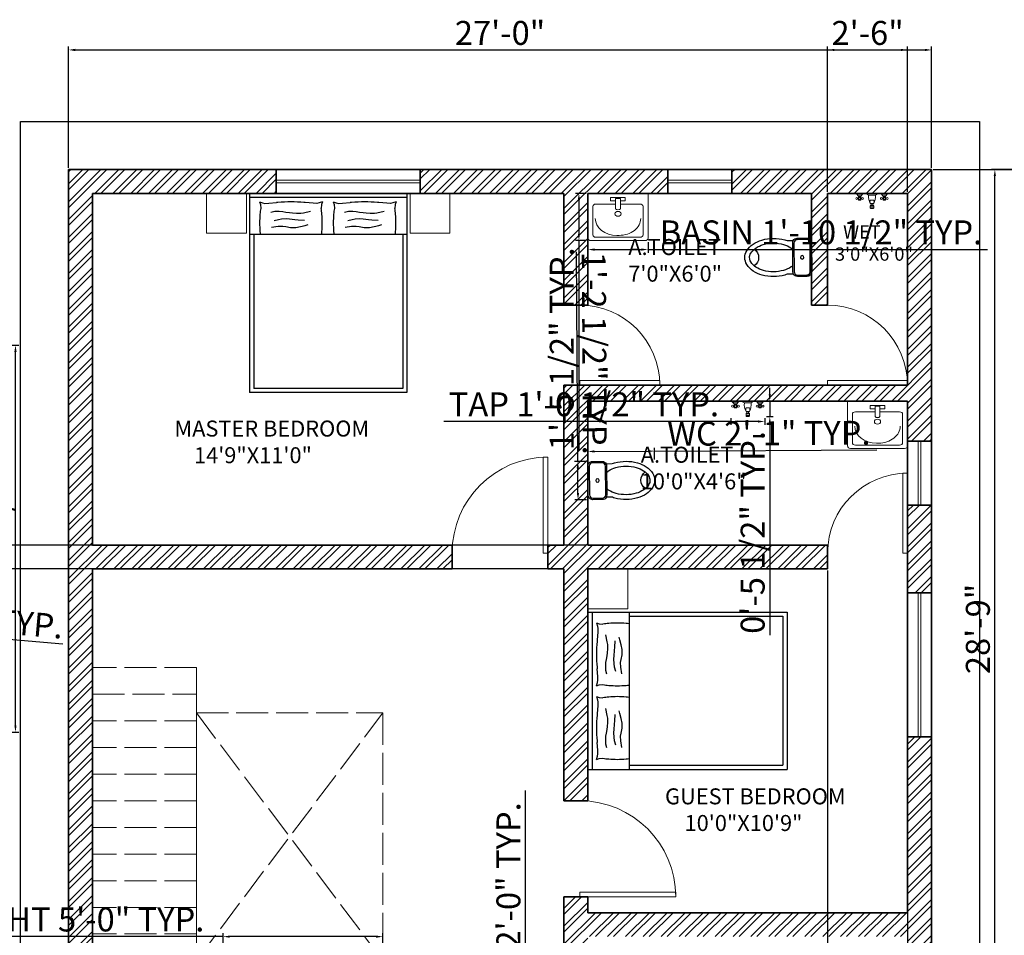
# Model space of a CAD drawing. Units: inches. Extents: x 638 to 1853, y 4393 to 5041.
# Tile 5 of 6: x 1072 to 1441, y 4619 to 4962. Entities that reach past the tile are written whole.
import ezdxf

# ---------------------------------------------------------------- set-up
doc = ezdxf.new("R2010")
doc.units = ezdxf.units.IN
doc.linetypes.add('ACAD_ISO02W100', pattern=[15, 12, -3])
for name, color, linetype, lineweight in [('A-ANNO-DIMS', 2, 'Continuous', 18), ('A-AREA-IDEN', 7, 'Continuous', 18), ('A-DOOR', 4, 'Continuous', 18), ('A-FLOR-FIXT', 9, 'Continuous', 18), ('A-FLOR-STRS', 7, 'Continuous', 18), ('A-FLOR-STRS-HIDN', 7, 'ACAD_ISO02W100', 18), ('A-FURN', 26, 'Continuous', 13), ('A-GLAZ', 5, 'Continuous', 18), ('A-WALL', 7, 'Continuous', 35), ('A-WALL-PATT', 251, 'Continuous', 13), ('C-PROP', 7, 'Continuous', 25)]:
    doc.layers.add(name, color=color, linetype=linetype, lineweight=lineweight)
for name, color, linetype in [('SANTEH', 7, 'Continuous'), ('supurgelik', 31, 'Continuous'), ('TASLAR', 32, 'Continuous')]:
    doc.layers.add(name, color=color, linetype=linetype)
doc.styles.get("Standard").update_dxf_attribs({"font": 'arial.ttf'})
doc.dimstyles.new('ISO-25', dxfattribs={"dimtxt": 9, "dimasz": 2.5, "dimexe": 1.25, "dimexo": 0.625, "dimtad": 1, "dimdec": 1, "dimlunit": 3, "dimtxsty": 'Standard', "dimcen": 2.5, "dimadec": 0, "dimazin": 0, "dimtfac": 1, "dimtdec": 1, "dimtmove": 0, "dimatfit": 3, "dimfxl": 1, "dimarcsym": 0})

# ---------------------------------------------------------------- blocks, each defined once
blk = doc.blocks.new('*U2')
for p, q in [((0, 0), (0, -6)), ((-36, 0), (-36, -6))]:
    blk.add_line(p, q)
blk.add_lwpolyline([(0, 0), (0, 36), (-1.75, 36), (-1.75, 0)], close=True)
blk.add_arc((0, 0), 36, 90, 180)
blk = doc.blocks.new('*U3')
for p, q in [((-30, 0), (-30, -6)), ((0, 0), (0, -6))]:
    blk.add_line(p, q)
blk.add_lwpolyline([(0, 0), (0, 30), (-1.75, 30), (-1.75, 0)], close=True)
blk.add_arc((0, 0), 30, 90, 180)
blk = doc.blocks.new('hgjgh')
at = {"layer": 'supurgelik'}
for p, q in [((85993.81, -4751.89), (85843.81, -4751.89)), ((85853.26, -4756.05), (85856.29, -4757)), ((85853.26, -4756.05), (85854.18, -4758.49)), ((85854.18, -4758.49), (85854.49, -4762.19)), ((85856.29, -4757), (85858.52, -4757.5)), ((85858.52, -4757.5), (85862.12, -4757.37)), ((85862.12, -4757.37), (85869.57, -4756.72)), ((85904.4, -4757.37), (85896.95, -4756.72)), ((85908, -4757.5), (85904.4, -4757.37)), ((85910.23, -4757), (85908, -4757.5)), ((85913.26, -4756.05), (85910.23, -4757)), ((85912.34, -4758.49), (85912.03, -4762.19)), ((85913.26, -4756.05), (85912.34, -4758.49)), ((85923.48, -4756.05), (85926.51, -4757)), ((85923.48, -4756.05), (85924.4, -4758.49)), ((85924.4, -4758.49), (85924.71, -4762.19)), ((85926.51, -4757), (85928.74, -4757.5)), ((85928.74, -4757.5), (85932.34, -4757.37)), ((85932.34, -4757.37), (85939.79, -4756.72)), ((85974.62, -4757.37), (85967.17, -4756.72)), ((85978.22, -4757.5), (85974.62, -4757.37)), ((85980.45, -4757), (85978.22, -4757.5)), ((85983.48, -4756.05), (85980.45, -4757)), ((85982.56, -4758.49), (85982.25, -4762.19)), ((85983.48, -4756.05), (85982.56, -4758.49)), ((85864.23, -4765.86), (85867.95, -4764.99)), ((85867.95, -4764.99), (85871.91, -4764.87)), ((85871.91, -4764.87), (85875.39, -4765.12)), ((85875.39, -4765.12), (85878.49, -4765.74)), ((85878.49, -4765.74), (85881.96, -4766.23)), ((85881.96, -4766.23), (85884.81, -4766.61)), ((85884.81, -4766.61), (85888.65, -4766.85)), ((85888.65, -4766.85), (85892.62, -4766.85)), ((85892.62, -4766.85), (85895.1, -4766.36)), ((85895.1, -4766.36), (85901.8, -4764.87)), ((85934.44, -4765.86), (85938.16, -4764.99)), ((85938.16, -4764.99), (85942.13, -4764.87)), ((85942.13, -4764.87), (85945.6, -4765.12)), ((85945.6, -4765.12), (85948.7, -4765.74)), ((85948.7, -4765.74), (85952.18, -4766.23)), ((85952.18, -4766.23), (85955.03, -4766.61)), ((85955.03, -4766.61), (85958.87, -4766.85)), ((85958.87, -4766.85), (85962.84, -4766.85)), ((85962.84, -4766.85), (85965.32, -4766.36)), ((85965.32, -4766.36), (85972.02, -4764.87)), ((85871.29, -4773.05), (85867.33, -4774.04)), ((85870.92, -4779.28), (85875.39, -4779.03)), ((85874.27, -4772.55), (85871.29, -4773.05)), ((85878.86, -4772.3), (85874.27, -4772.55)), ((85875.39, -4779.03), (85878.24, -4779.65)), ((85881.96, -4772.55), (85878.86, -4772.3)), ((85887.04, -4773.05), (85881.96, -4772.55)), ((85890.14, -4773.3), (85887.04, -4773.05)), ((85896.09, -4773.67), (85890.14, -4773.3)), ((85892.37, -4779.65), (85896.96, -4778.41)), ((85896.96, -4778.41), (85899.69, -4777.54)), ((85941.51, -4773.05), (85937.54, -4774.04)), ((85941.14, -4779.28), (85945.6, -4779.03)), ((85944.49, -4772.55), (85941.51, -4773.05)), ((85949.08, -4772.3), (85944.49, -4772.55)), ((85945.6, -4779.03), (85948.46, -4779.65)), ((85952.18, -4772.55), (85949.08, -4772.3)), ((85957.26, -4773.05), (85952.18, -4772.55)), ((85960.36, -4773.3), (85957.26, -4773.05)), ((85966.31, -4773.67), (85960.36, -4773.3)), ((85962.59, -4779.65), (85967.18, -4778.41)), ((85967.18, -4778.41), (85969.91, -4777.54)), ((85993.81, -4787.2), (85843.81, -4787.2)), ((85847.81, -4787.2), (85847.81, -4933.89)), ((85864.72, -4780.15), (85870.92, -4779.28)), ((85878.24, -4779.65), (85882.95, -4780.4)), ((85882.95, -4780.4), (85887.91, -4780.4)), ((85887.91, -4780.4), (85892.37, -4779.65)), ((85934.94, -4780.15), (85941.14, -4779.28)), ((85948.46, -4779.65), (85953.17, -4780.4)), ((85953.17, -4780.4), (85958.13, -4780.4)), ((85958.13, -4780.4), (85962.59, -4779.65)), ((85989.81, -4787.2), (85989.81, -4933.89)), ((85989.81, -4933.89), (85847.81, -4933.89))]:
    blk.add_line(p, q, dxfattribs=at)
for centre, radius, start, end in [((85877.36, -4828.49), 72.19, 95.13619, 96.19323), ((85883.26, -4894.18), 138.14, 90, 95.13619), ((85883.26, -4894.18), 138.14, 84.86381, 90), ((85889.16, -4828.49), 72.19, 83.80677, 84.86381), ((85947.57, -4828.49), 72.19, 95.13619, 96.19323), ((85953.48, -4894.18), 138.14, 90, 95.13619), ((85953.48, -4894.18), 138.14, 84.86381, 90), ((85959.38, -4828.49), 72.19, 83.80677, 84.86381), ((85954.09, -4776.05), 100.71, 175.30047, 180), ((85905.8, -4772.08), 52.26, 169.08956, 175.30047), ((85860.72, -4772.08), 52.26, 4.69953, 10.91044), ((85812.43, -4776.05), 100.71, 0, 4.69953), ((86024.31, -4776.05), 100.71, 175.30047, 180), ((85976.02, -4772.08), 52.26, 169.08956, 175.30047), ((85930.94, -4772.08), 52.26, 4.69953, 10.91044), ((85882.65, -4776.05), 100.71, 0, 4.69953), ((85954.09, -4776.05), 100.71, 180, 184.69953), ((85812.43, -4776.05), 100.71, 355.30047, 0), ((86024.31, -4776.05), 100.71, 180, 184.69953), ((85882.65, -4776.05), 100.71, 355.30047, 0), ((85905.8, -4780.02), 52.26, 184.69953, 187.89725), ((85860.72, -4780.02), 52.26, 352.10275, 355.30047), ((85976.02, -4780.02), 52.26, 184.69953, 187.89725), ((85930.94, -4780.02), 52.26, 352.10275, 355.30047)]:
    blk.add_arc(centre, radius, start, end, dxfattribs=at)
at = {"layer": 'TASLAR'}
for p, q in [((85843.81, -4747.89), (85843.81, -4937.89)), ((85993.81, -4747.89), (85843.81, -4747.89)), ((85993.81, -4747.89), (85993.81, -4937.89)), ((85993.81, -4937.89), (85843.81, -4937.89))]:
    blk.add_line(p, q, dxfattribs=at)
blk = doc.blocks.new('Rac7')
at = {"color": 0}
for p, q in [((-39500.6, -24232.1), (-39500.6, -23829.6)), ((-39473.6, -23808.4), (-38988.3, -23808.4)), ((-39456.5, -23859.1), (-39456.5, -24114.9)), ((-39032.4, -23838), (-39429.6, -23838)), ((-39221.1, -23854.9), (-39240.8, -23854.9)), ((-39005.4, -24114.9), (-39005.4, -23859.1)), ((-39005.4, -23859.1), (-39005.4, -23859.1)), ((-38961.3, -23829.6), (-38961.3, -24232.1)), ((-39252.5, -24185.9), (-39252.5, -24093.6)), ((-39209.4, -24185.9), (-39209.4, -24093.6)), ((-39429.6, -24136.1), (-39252.5, -24136.1)), ((-39297, -24164), (-39252.5, -24164)), ((-39297, -24193.5), (-39297, -24164)), ((-39164.9, -24193.5), (-39297, -24193.5)), ((-39252.5, -24185.9), (-39209.4, -24185.9)), ((-39209.4, -24136.1), (-39032.4, -24136.1)), ((-39209.4, -24164), (-39164.9, -24164)), ((-39164.9, -24164), (-39164.9, -24193.5)), ((-38961.3, -24232.1), (-39500.6, -24232.1))]:
    blk.add_line(p, q, dxfattribs=at)
at = {"color": 0, "extrusion": (0, 0, -1)}
for centre, major_axis, start_param, end_param in [((-39473.6, -23829.6), (-27, 0), 0, 1.570796), ((-39429.6, -23859.1), (-27, 0), 0, 1.570796), ((-39240.8, -24007.4), (-194.1, 0), 0, 1.570796), ((-39221.1, -24007.4), (-194.1, 0), 1.570796, 3.141593), ((-39032.4, -23859.1), (-27, 0), 1.570796, 3.141593), ((-38988.3, -23829.6), (-27, 0), 1.570796, 3.141593), ((-39429.6, -24114.9), (-27, 0), -1.570796, 0), ((-39231, -24104), (-25.3, 0), 0.552816, 2.588777), ((-39032.4, -24114.9), (-27, 0), -3.141593, -1.570796)]:
    blk.add_ellipse(centre, major_axis=major_axis, ratio=0.785714, start_param=start_param, end_param=end_param, dxfattribs=at)
blk.add_ellipse((-39231, -24048), major_axis=(-27.9, 0), ratio=0.785714, dxfattribs=at)
blk = doc.blocks.new('K10-44')
at = {"layer": 'SANTEH'}
for points in [[(-182, 223, 0.020439), (-174, 198), (-174, 135, 0.262987), (-198, 92), (-198, -8, 0.414214), (-148, -58), (152, -58, 0.414214), (202, -8), (202, 92, 0.262987), (178, 135), (178, 198, 0.020439), (186, 223, 0.067459), (202, 342, 0.067459), (186, 461, 0.079812), (143, 554, 0.107118), (74, 621, 0.139889), (2, 642, 0.139889), (-70, 621, 0.107118), (-140, 554, 0.079812), (-182, 461, 0.067459), (-198, 342, 0.067459)], [(-148, 127), (152, 127, -0.414214), (187, 92), (187, -8, -0.414214), (152, -43), (-148, -43, -0.414214), (-183, -8), (-183, 92, -0.414214)]]:
    blk.add_lwpolyline(points, format="xyb", close=True, dxfattribs=at)
for points in [[(90, 142, 0.027307), (102, 158, 0.079812), (137, 236, 0.067459), (152, 342, 0.067459), (137, 448, 0.079812), (102, 526, 0.107118), (47, 579, 0.139889), (2, 592, 0.139889), (-44, 579, 0.107118), (-98, 526, 0.079812), (-134, 448, 0.067459), (-148, 342, 0.067459), (-134, 236, 0.079812), (-98, 158, 0.027307), (-86, 142, 0.139889)], [(-174, 135, -0.136371), (-148, 142), (152, 142, -0.136371), (178, 135)]]:
    blk.add_lwpolyline(points, format="xyb", dxfattribs=at)
blk.add_circle((2, 42), 18.3, dxfattribs=at)
blk.add_arc((2, 602), 105, 213.8994, 326.1006, dxfattribs=at)
blk = doc.blocks.new('Faucet - Bathroom front')
for p, q in [((-0.5, 4.25), (0.5, 4.25)), ((0.5, 3.75), (-0.5, 3.75)), ((-0.5, 3), (0.5, 3)), ((-0.25, 3), (-0.25, 3.5)), ((0.25, 3.5), (0.25, 3)), ((-5, 0), (-2.25, 0)), ((-4.5087, 0.25), (-2.7408, 0.25)), ((-4, 1.625), (-4.25, 1.625)), ((-4, 1.375), (-4.25, 1.375)), ((-3.1442, 0.75), (-4.0979, 0.75)), ((-3.25, 1.625), (-3, 1.625)), ((-3.25, 1.375), (-3, 1.375)), ((-1.5, 0), (1.5, 0)), ((-1, 0.5), (1, 0.5)), ((0.5, 2), (-0.5, 2)), ((2.25, 0), (5, 0)), ((2.7413, 0.25), (4.5092, 0.25)), ((3.25, 1.625), (3, 1.625)), ((3.25, 1.375), (3, 1.375)), ((4.1058, 0.75), (3.1521, 0.75)), ((4, 1.625), (4.25, 1.625)), ((4, 1.375), (4.25, 1.375))]:
    blk.add_line(p, q)
for points in [[(-0.5, 3.75), (-0.5, 4.25)], [(-0.25, 4.5), (0.25, 4.5)], [(0.25, 3.5), (-0.25, 3.5)], [(0.5, 4.25), (0.5, 3.75)]]:
    blk.add_lwpolyline(points)
for points in [[(-4, 1), (-4, 2), (-3.25, 2), (-3.25, 1)], [(3.25, 1), (3.25, 2), (4, 2), (4, 1)]]:
    blk.add_lwpolyline(points, close=True)
for centre in [(-4.5, 1.5), (-3.625, 1.5), (-2.75, 1.5), (2.75, 1.5), (3.625, 1.5), (4.5, 1.5)]:
    blk.add_circle(centre, 0.2795)
for centre, radius, start, end in [((3, 1), 4.0311, 150.2551, 187.125), ((0.6413, 2.5), 1.246, 156.3417, 203.6583), ((-0.2575, 4.2575), 0.2426, 88.22243, 181.7776), ((-0.2575, 3.7425), 0.2426, 178.2224, 271.7776), ((0.2575, 4.2575), 0.2426, 358.2224, 91.77757), ((0.2575, 3.7425), 0.2426, 268.2224, 1.777565), ((-3, 1), 4.0311, 352.875, 29.74488), ((-0.6413, 2.5), 1.246, 336.3417, 23.65835), ((-5.375, 1.375), 1.4252, 285.2551, 344.7449), ((-1.875, 1.375), 1.4252, 195.2551, 254.7449), ((-0.7962, -0.2038), 0.7327, 106.1502, 163.8498), ((0.7962, -0.2038), 0.7327, 16.1502, 73.84979), ((1.875, 1.375), 1.4252, 285.2551, 344.7449), ((5.375, 1.375), 1.4252, 195.2551, 254.7449)]:
    blk.add_arc(centre, radius, start, end)
blk = doc.blocks.new('BED-NIGHTSTAND-15')
blk.add_lwpolyline([(0, 14.98), (14.98, 14.98), (14.98, 0), (0, 0)], close=True)
blk = doc.blocks.new('WINDOW-GLAZING-24IN')
for p, q in [((0, 24), (0, 0)), ((1, 24), (1, 0))]:
    blk.add_line(p, q)
blk = doc.blocks.new('WINDOW-GLAZING-54IN')
for p, q in [((0, 1), (54, 1)), ((0, 0), (54, 0))]:
    blk.add_line(p, q)
blk = doc.blocks.new('STAIR-WELL-OPENING')
for p, q in [((0, 93), (70, 0)), ((0, 0), (70, 93))]:
    blk.add_line(p, q)
blk.add_lwpolyline([(0, 93), (70, 93), (70, 0), (0, 0)], close=True)
blk = doc.blocks.new('STAIR-RUN-BEYOND')
for p, q in [((39, 100), (0, 100)), ((0, 90), (39, 90)), ((39, 80), (0, 80)), ((39, 70), (0, 70)), ((39, 60), (0, 60)), ((39, 50), (0, 50)), ((39, 40), (0, 40)), ((39, 30), (0, 30)), ((39, 20), (0, 20)), ((39, 10), (0, 10)), ((39, 0), (0, 0)), ((39, 0), (0, 0))]:
    blk.add_line(p, q)
blk = doc.blocks.new('*D40')
at = {"layer": 'A-ANNO-DIMS', "color": 0, "lineweight": -2, "transparency": 16777216}
for p, q in [((1285.04, 4797.16), (1285.01, 4801.55)), ((1287.52, 4800.31), (1307.62, 4800.43)), ((1310.13, 4797.3), (1310.11, 4801.69)), ((1310.12, 4800.44), (1393.53, 4800.92))]:
    blk.add_line(p, q, dxfattribs=at)
at = {"layer": 'A-ANNO-DIMS', "color": 0, "transparency": 16777216}
for points in [[(1287.52, 4800.73), (1287.52, 4799.9), (1285.02, 4800.3)], [(1307.61, 4800.84), (1307.62, 4800.01), (1310.12, 4800.44)]]:
    blk.add_solid(points, dxfattribs=at)
at = {"layer": 'Defpoints', "color": 0, "transparency": 16777216}
for p in [(1310.12, 4800.44), (1285.04, 4796.53), (1310.14, 4796.68)]:
    blk.add_point(p, dxfattribs=at)
at = {"layer": 'A-ANNO-DIMS', "color": 0, "transparency": 16777216, "insert": (1353.04, 4805.97), "char_height": 9, "attachment_point": 5, "rotation": 0.328}
blk.add_mtext('WC 2\'-1" TYP.', dxfattribs=at)
blk = doc.blocks.new('*D41')
at = {"layer": 'A-ANNO-DIMS', "color": 0, "lineweight": -2, "transparency": 16777216}
for p, q in [((1281.28, 4796.51), (1280.83, 4875.25)), ((1284.42, 4796.53), (1280.03, 4796.51)), ((1281.34, 4784.67), (1281.29, 4794.01)), ((1284.5, 4782.19), (1280.11, 4782.16))]:
    blk.add_line(p, q, dxfattribs=at)
at = {"layer": 'A-ANNO-DIMS', "color": 0, "transparency": 16777216}
for points in [[(1281.71, 4794.02), (1280.87, 4794.01), (1281.28, 4796.51)], [(1281.76, 4784.67), (1280.93, 4784.67), (1281.36, 4782.17)]]:
    blk.add_solid(points, dxfattribs=at)
at = {"layer": 'Defpoints', "color": 0, "transparency": 16777216}
for p in [(1281.28, 4796.51), (1285.04, 4796.53), (1285.12, 4782.19)]:
    blk.add_point(p, dxfattribs=at)
at = {"layer": 'A-ANNO-DIMS', "color": 0, "transparency": 16777216, "insert": (1286.32, 4837.16), "char_height": 9, "attachment_point": 5, "rotation": 270.328}
blk.add_mtext('1\'-2 1/2" TYP.', dxfattribs=at)
blk = doc.blocks.new('*D42')
at = {"layer": 'A-ANNO-DIMS', "color": 0, "lineweight": -2, "transparency": 16777216}
for p, q in [((1338.71, 4811.55), (1230.96, 4811.55)), ((1338.71, 4812.83), (1338.71, 4810.3)), ((1348.95, 4811.55), (1341.21, 4811.55)), ((1351.45, 4812.83), (1351.45, 4810.3))]:
    blk.add_line(p, q, dxfattribs=at)
at = {"layer": 'A-ANNO-DIMS', "color": 0, "transparency": 16777216}
for points in [[(1341.21, 4811.96), (1341.21, 4811.13), (1338.71, 4811.55)], [(1348.95, 4811.96), (1348.95, 4811.13), (1351.45, 4811.55)]]:
    blk.add_solid(points, dxfattribs=at)
at = {"layer": 'Defpoints', "color": 0, "transparency": 16777216}
for p in [(1338.71, 4813.46), (1351.45, 4813.46), (1338.71, 4811.55)]:
    blk.add_point(p, dxfattribs=at)
at = {"layer": 'A-ANNO-DIMS', "color": 0, "transparency": 16777216, "insert": (1283.58, 4816.83), "char_height": 9, "attachment_point": 5}
blk.add_mtext('TAP 1\'-0 1/2" TYP.', dxfattribs=at)
blk = doc.blocks.new('*D43')
at = {"layer": 'A-ANNO-DIMS', "color": 0, "lineweight": -2, "transparency": 16777216}
for p, q in [((1353.36, 4821.69), (1353.36, 4824.19)), ((1352.08, 4819.19), (1354.61, 4819.19)), ((1353.36, 4819.19), (1353.36, 4813.46)), ((1352.08, 4813.46), (1354.61, 4813.46)), ((1353.36, 4810.96), (1353.36, 4731.38))]:
    blk.add_line(p, q, dxfattribs=at)
at = {"layer": 'A-ANNO-DIMS', "color": 0, "transparency": 16777216}
for points in [[(1352.95, 4821.69), (1353.78, 4821.69), (1353.36, 4819.19)], [(1352.95, 4810.96), (1353.78, 4810.96), (1353.36, 4813.46)]]:
    blk.add_solid(points, dxfattribs=at)
at = {"layer": 'Defpoints', "color": 0, "transparency": 16777216}
for p in [(1351.45, 4819.19), (1351.45, 4813.46), (1353.36, 4813.46)]:
    blk.add_point(p, dxfattribs=at)
at = {"layer": 'A-ANNO-DIMS', "color": 0, "transparency": 16777216, "insert": (1348.09, 4769.92), "char_height": 9, "attachment_point": 5, "rotation": 90}
blk.add_mtext('0\'-5 1/2" TYP.', dxfattribs=at)
blk = doc.blocks.new('*D48')
at = {"layer": 'A-ANNO-DIMS', "color": 0, "lineweight": -2, "transparency": 16777216}
for p, q in [((1285.08, 4878.85), (1285.08, 4874.84)), ((1287.58, 4876.09), (1305.14, 4876.09)), ((1307.64, 4878.85), (1307.64, 4874.84)), ((1307.64, 4876.09), (1435.04, 4876.09))]:
    blk.add_line(p, q, dxfattribs=at)
at = {"layer": 'A-ANNO-DIMS', "color": 0, "transparency": 16777216}
for points in [[(1287.58, 4876.51), (1287.58, 4875.67), (1285.08, 4876.09)], [(1305.14, 4876.51), (1305.14, 4875.67), (1307.64, 4876.09)]]:
    blk.add_solid(points, dxfattribs=at)
at = {"layer": 'Defpoints', "color": 0, "transparency": 16777216}
for p in [(1285.08, 4879.47), (1307.64, 4879.47), (1307.64, 4876.09)]:
    blk.add_point(p, dxfattribs=at)
at = {"layer": 'A-ANNO-DIMS', "color": 0, "transparency": 16777216, "insert": (1372.59, 4881.37), "char_height": 9, "attachment_point": 5}
blk.add_mtext('BASIN 1\'-10 1/2" TYP.', dxfattribs=at)
blk = doc.blocks.new('*D49')
at = {"layer": 'A-ANNO-DIMS', "color": 0, "lineweight": -2, "transparency": 16777216}
for p, q in [((1284.46, 4897.19), (1280.45, 4897.19)), ((1281.7, 4894.69), (1281.7, 4881.97)), ((1284.46, 4879.47), (1280.45, 4879.47)), ((1281.7, 4879.47), (1281.7, 4800.74))]:
    blk.add_line(p, q, dxfattribs=at)
at = {"layer": 'A-ANNO-DIMS', "color": 0, "transparency": 16777216}
for points in [[(1281.28, 4894.69), (1282.11, 4894.69), (1281.7, 4897.19)], [(1281.28, 4881.97), (1282.11, 4881.97), (1281.7, 4879.47)]]:
    blk.add_solid(points, dxfattribs=at)
at = {"layer": 'Defpoints', "color": 0, "transparency": 16777216}
for p in [(1285.08, 4897.19), (1281.7, 4879.47), (1285.08, 4879.47)]:
    blk.add_point(p, dxfattribs=at)
at = {"layer": 'A-ANNO-DIMS', "color": 0, "transparency": 16777216, "insert": (1276.42, 4838.86), "char_height": 9, "attachment_point": 5, "rotation": 90}
blk.add_mtext('1\'-5 1/2" TYP.', dxfattribs=at)
blk = doc.blocks.new('*D51')
at = {"layer": 'A-ANNO-DIMS', "color": 0, "lineweight": -2, "transparency": 16777216}
for p, q in [((999.03, 4734.62), (999.24, 4737.06)), ((1001.62, 4735.59), (1006.2, 4735.19)), ((1008.59, 4733.79), (1008.8, 4736.22)), ((1008.69, 4734.98), (1087.97, 4728.04))]:
    blk.add_line(p, q, dxfattribs=at)
at = {"layer": 'A-ANNO-DIMS', "color": 0, "transparency": 16777216}
for points in [[(1001.66, 4736.01), (1001.59, 4735.18), (999.13, 4735.81)], [(1006.24, 4735.61), (1006.17, 4734.78), (1008.69, 4734.98)]]:
    blk.add_solid(points, dxfattribs=at)
at = {"layer": 'Defpoints', "color": 0, "transparency": 16777216}
for p in [(998.97, 4734), (1008.54, 4733.16), (1008.69, 4734.98)]:
    blk.add_point(p, dxfattribs=at)
at = {"layer": 'A-ANNO-DIMS', "color": 0, "transparency": 16777216, "insert": (1050.04, 4736.66), "char_height": 9, "attachment_point": 5, "rotation": 355}
blk.add_mtext('0\'-9 1/2" TYP.', dxfattribs=at)
blk = doc.blocks.new('*D56')
at = {"layer": 'A-ANNO-DIMS', "color": 0, "lineweight": -2, "transparency": 16777216}
for p, q in [((1261.68, 4538.69), (1261.68, 4673.01)), ((1258.71, 4538.69), (1262.93, 4538.69)), ((1261.68, 4517.19), (1261.68, 4536.19)), ((1258.71, 4514.69), (1262.93, 4514.69))]:
    blk.add_line(p, q, dxfattribs=at)
at = {"layer": 'A-ANNO-DIMS', "color": 0, "transparency": 16777216}
for points in [[(1261.26, 4536.19), (1262.1, 4536.19), (1261.68, 4538.69)], [(1261.26, 4517.19), (1262.1, 4517.19), (1261.68, 4514.69)]]:
    blk.add_solid(points, dxfattribs=at)
at = {"layer": 'Defpoints', "color": 0, "transparency": 16777216}
for p in [(1258.08, 4538.69), (1261.68, 4538.69), (1258.08, 4514.69)]:
    blk.add_point(p, dxfattribs=at)
at = {"layer": 'A-ANNO-DIMS', "color": 0, "transparency": 16777216, "insert": (1256.4, 4607.1), "char_height": 9, "attachment_point": 5, "rotation": 90}
blk.add_mtext('DOOR LEAF 2\'-0" TYP.', dxfattribs=at)
blk = doc.blocks.new('*D58')
at = {"layer": 'A-ANNO-DIMS', "color": 0, "lineweight": -2, "transparency": 16777216}
for p, q in [((1148.08, 4618.19), (1000.8, 4618.19)), ((1148.08, 4609.82), (1148.08, 4619.44)), ((1205.58, 4618.19), (1150.58, 4618.19)), ((1208.08, 4609.82), (1208.08, 4619.44))]:
    blk.add_line(p, q, dxfattribs=at)
at = {"layer": 'A-ANNO-DIMS', "color": 0, "transparency": 16777216}
for points in [[(1150.58, 4618.61), (1150.58, 4617.78), (1148.08, 4618.19)], [(1205.58, 4618.61), (1205.58, 4617.78), (1208.08, 4618.19)]]:
    blk.add_solid(points, dxfattribs=at)
at = {"layer": 'Defpoints', "color": 0, "transparency": 16777216}
for p in [(1148.08, 4618.19), (1148.08, 4609.19), (1208.08, 4609.19)]:
    blk.add_point(p, dxfattribs=at)
at = {"layer": 'A-ANNO-DIMS', "color": 0, "transparency": 16777216, "insert": (1073.19, 4623.47), "char_height": 9, "attachment_point": 5}
blk.add_mtext('STAIR FLIGHT 5\'-0" TYP.', dxfattribs=at)
blk = doc.blocks.new('*D83')
at = {"layer": 'A-ANNO-DIMS', "color": 0, "lineweight": -2, "transparency": 16777216}
for p, q in [((1016.97, 4840.19), (1071.42, 4840.19)), ((1070.17, 4697.42), (1070.17, 4837.69)), ((1016.97, 4694.92), (1071.42, 4694.92))]:
    blk.add_line(p, q, dxfattribs=at)
at = {"layer": 'A-ANNO-DIMS', "color": 0, "transparency": 16777216}
for points in [[(1069.75, 4837.69), (1070.58, 4837.69), (1070.17, 4840.19)], [(1069.75, 4697.42), (1070.58, 4697.42), (1070.17, 4694.92)]]:
    blk.add_solid(points, dxfattribs=at)
at = {"layer": 'Defpoints', "color": 0, "transparency": 16777216}
for p in [(1016.34, 4840.19), (1070.17, 4840.19), (1016.34, 4694.92)]:
    blk.add_point(p, dxfattribs=at)
at = {"layer": 'A-ANNO-DIMS', "color": 0, "transparency": 16777216, "insert": (1064.89, 4767.56), "char_height": 9, "attachment_point": 5, "rotation": 90}
blk.add_mtext('12\'-1 1/2"', dxfattribs=at)
blk = doc.blocks.new('*D88')
at = {"layer": 'A-ANNO-DIMS', "color": 0, "lineweight": -2, "transparency": 16777216}
for p, q in [((1090.08, 4906.82), (1090.08, 4952.27)), ((1092.58, 4951.02), (1411.58, 4951.02)), ((1414.08, 4906.82), (1414.08, 4952.27))]:
    blk.add_line(p, q, dxfattribs=at)
at = {"layer": 'A-ANNO-DIMS', "color": 0, "transparency": 16777216}
for points in [[(1092.58, 4951.44), (1092.58, 4950.6), (1090.08, 4951.02)], [(1411.58, 4951.44), (1411.58, 4950.6), (1414.08, 4951.02)]]:
    blk.add_solid(points, dxfattribs=at)
at = {"layer": 'Defpoints', "color": 0, "transparency": 16777216}
for p in [(1414.08, 4951.02), (1090.08, 4906.19), (1414.08, 4906.19)]:
    blk.add_point(p, dxfattribs=at)
at = {"layer": 'A-ANNO-DIMS', "color": 0, "transparency": 16777216, "insert": (1252.08, 4956.24), "char_height": 9, "attachment_point": 5}
blk.add_mtext('27\'-0"', dxfattribs=at)
blk = doc.blocks.new('*D89')
at = {"layer": 'A-ANNO-DIMS', "color": 0, "lineweight": -2, "transparency": 16777216}
for p, q in [((1414.71, 4906.19), (1460.16, 4906.19)), ((1458.91, 4458.69), (1458.91, 4903.69)), ((1414.71, 4456.19), (1460.16, 4456.19))]:
    blk.add_line(p, q, dxfattribs=at)
at = {"layer": 'A-ANNO-DIMS', "color": 0, "transparency": 16777216}
for points in [[(1458.49, 4903.69), (1459.32, 4903.69), (1458.91, 4906.19)], [(1458.49, 4458.69), (1459.32, 4458.69), (1458.91, 4456.19)]]:
    blk.add_solid(points, dxfattribs=at)
at = {"layer": 'Defpoints', "color": 0, "transparency": 16777216}
for p in [(1414.08, 4906.19), (1458.91, 4906.19), (1414.08, 4456.19)]:
    blk.add_point(p, dxfattribs=at)
at = {"layer": 'A-ANNO-DIMS', "color": 0, "transparency": 16777216, "insert": (1453.68, 4681.19), "char_height": 9, "attachment_point": 5, "rotation": 90}
blk.add_mtext('37\'-6"', dxfattribs=at)
blk = doc.blocks.new('*D91')
at = {"layer": 'A-ANNO-DIMS', "color": 0, "lineweight": -2, "transparency": 16777216}
for p, q in [((1375.08, 4897.82), (1375.08, 4952.27)), ((1377.58, 4951.02), (1402.58, 4951.02)), ((1405.08, 4897.82), (1405.08, 4952.27))]:
    blk.add_line(p, q, dxfattribs=at)
at = {"layer": 'A-ANNO-DIMS', "color": 0, "transparency": 16777216}
for points in [[(1377.58, 4951.44), (1377.58, 4950.6), (1375.08, 4951.02)], [(1402.58, 4951.44), (1402.58, 4950.6), (1405.08, 4951.02)]]:
    blk.add_solid(points, dxfattribs=at)
at = {"layer": 'Defpoints', "color": 0, "transparency": 16777216}
for p in [(1405.08, 4951.02), (1375.08, 4897.19), (1405.08, 4897.19)]:
    blk.add_point(p, dxfattribs=at)
at = {"layer": 'A-ANNO-DIMS', "color": 0, "transparency": 16777216, "insert": (1390.08, 4956.24), "char_height": 9, "attachment_point": 5}
blk.add_mtext('2\'-6"', dxfattribs=at)
blk = doc.blocks.new('*D92')
at = {"layer": 'A-ANNO-DIMS', "color": 0, "lineweight": -2, "transparency": 16777216}
for p, q in [((1375.08, 4755.57), (1375.08, 4416.12)), ((1405.08, 4755.57), (1405.08, 4416.12)), ((1377.58, 4417.37), (1402.58, 4417.37))]:
    blk.add_line(p, q, dxfattribs=at)
at = {"layer": 'A-ANNO-DIMS', "color": 0, "transparency": 16777216}
for points in [[(1377.58, 4417.79), (1377.58, 4416.95), (1375.08, 4417.37)], [(1402.58, 4417.79), (1402.58, 4416.95), (1405.08, 4417.37)]]:
    blk.add_solid(points, dxfattribs=at)
at = {"layer": 'Defpoints', "color": 0, "transparency": 16777216}
for p in [(1375.08, 4756.19), (1405.08, 4756.19), (1405.08, 4417.37)]:
    blk.add_point(p, dxfattribs=at)
at = {"layer": 'A-ANNO-DIMS', "color": 0, "transparency": 16777216, "insert": (1390.08, 4422.59), "char_height": 9, "attachment_point": 5}
blk.add_mtext('2\'-6"', dxfattribs=at)
blk = doc.blocks.new('*D93')
at = {"layer": 'A-ANNO-DIMS', "color": 0, "lineweight": -2, "transparency": 16777216}
for p, q in [((1045.26, 4765.19), (1045.26, 4792.87)), ((1284.46, 4765.19), (1044.01, 4765.19)), ((1045.26, 4758.69), (1045.26, 4762.69)), ((1275.46, 4756.19), (1044.01, 4756.19))]:
    blk.add_line(p, q, dxfattribs=at)
at = {"layer": 'A-ANNO-DIMS', "color": 0, "transparency": 16777216}
for points in [[(1044.84, 4762.69), (1045.67, 4762.69), (1045.26, 4765.19)], [(1044.84, 4758.69), (1045.67, 4758.69), (1045.26, 4756.19)]]:
    blk.add_solid(points, dxfattribs=at)
at = {"layer": 'Defpoints', "color": 0, "transparency": 16777216}
for p in [(1045.26, 4765.19), (1285.08, 4765.19), (1276.08, 4756.19)]:
    blk.add_point(p, dxfattribs=at)
at = {"layer": 'A-ANNO-DIMS', "color": 0, "transparency": 16777216, "insert": (1040.04, 4780.28), "char_height": 9, "attachment_point": 5, "rotation": 90}
blk.add_mtext('0\'-9"', dxfattribs=at)
blk = doc.blocks.new('*D97')
at = {"layer": 'A-ANNO-DIMS', "color": 0, "lineweight": -2, "transparency": 16777216}
for p, q in [((1482.06, 4906.19), (1436.61, 4906.19)), ((1437.86, 4563.69), (1437.86, 4903.69)), ((1482.06, 4561.19), (1436.61, 4561.19))]:
    blk.add_line(p, q, dxfattribs=at)
at = {"layer": 'A-ANNO-DIMS', "color": 0, "transparency": 16777216}
for points in [[(1437.44, 4903.69), (1438.27, 4903.69), (1437.86, 4906.19)], [(1437.44, 4563.69), (1438.27, 4563.69), (1437.86, 4561.19)]]:
    blk.add_solid(points, dxfattribs=at)
at = {"layer": 'Defpoints', "color": 0, "transparency": 16777216}
for p in [(1437.86, 4906.19), (1482.68, 4906.19), (1482.68, 4561.19)]:
    blk.add_point(p, dxfattribs=at)
at = {"layer": 'A-ANNO-DIMS', "color": 0, "transparency": 16777216, "insert": (1432.64, 4733.69), "char_height": 9, "attachment_point": 5, "rotation": 90}
blk.add_mtext('28\'-9"', dxfattribs=at)

msp = doc.modelspace()

# ---------------------------------------------------------------- hatches: boundary and pattern name
at = {"layer": 'A-WALL-PATT', "transparency": 33554687}
h = msp.add_hatch(dxfattribs=at)
h.set_pattern_fill('ANSI32', color=256, scale=0.5)
h.set_pattern_definition([(45, (-45.7406, 0), (-3.367596, 3.367596), []), (45, (-43.4956, 0), (-3.367596, 3.367596), [])])
h.paths.add_polyline_path([(1414.08, 4693.19), (1405.08, 4693.19), (1405.08, 4627.19), (1285.08, 4627.19), (1285.08, 4633.19), (1282.08, 4633.19), (1276.08, 4633.19), (1276.08, 4612.19), (1282.08, 4612.19), (1285.08, 4612.19), (1285.08, 4618.19), (1405.08, 4618.19), (1405.08, 4465.19), (1381.08, 4465.19), (1381.08, 4456.19), (1414.08, 4456.19)])
h.paths.add_polyline_path([(1216.08, 4519.19), (1156.08, 4519.19), (1156.08, 4531.19), (1150.08, 4531.19), (1147.08, 4531.19), (1147.08, 4465.19), (1099.08, 4465.19), (1099.08, 4474.19), (1090.08, 4474.19), (1090.08, 4456.19), (1156.08, 4456.19), (1156.08, 4510.19), (1216.08, 4510.19)])
h.paths.add_polyline_path([(1285.08, 4576.19), (1276.08, 4576.19), (1276.08, 4519.19), (1258.08, 4519.19), (1258.08, 4517.69), (1258.08, 4514.69), (1258.08, 4510.19), (1276.08, 4510.19), (1276.08, 4456.19), (1309.08, 4456.19), (1309.08, 4465.19), (1285.08, 4465.19)])
h.paths.add_polyline_path([(1414.08, 4780.19), (1405.08, 4780.19), (1405.08, 4762.19), (1405.08, 4756.19), (1405.08, 4747.19), (1414.08, 4747.19)], flags=17)
h.paths.add_polyline_path([(1414.08, 4906.19), (1339.08, 4906.19), (1339.08, 4897.19), (1369.08, 4897.19), (1369.08, 4855.19), (1375.08, 4855.19), (1375.08, 4897.19), (1405.08, 4897.19), (1405.08, 4825.19), (1276.08, 4825.19), (1276.08, 4765.19), (1270.08, 4765.19), (1270.08, 4756.19), (1276.08, 4756.19), (1276.08, 4669.19), (1285.08, 4669.19), (1285.08, 4756.19), (1375.08, 4756.19), (1375.08, 4765.19), (1285.08, 4765.19), (1285.08, 4819.19), (1405.08, 4819.19), (1405.08, 4804.19), (1414.08, 4804.19)])
h.paths.add_polyline_path([(1315.08, 4906.19), (1222.08, 4906.19), (1222.08, 4897.19), (1233.28, 4897.19), (1276.08, 4897.19), (1276.08, 4855.19), (1282.08, 4855.19), (1285.08, 4855.19), (1285.08, 4897.19), (1307.64, 4897.19), (1315.08, 4897.19)])
h.paths.add_polyline_path([(1099.08, 4897.19), (1168.08, 4897.19), (1168.08, 4906.19), (1090.08, 4906.19), (1090.08, 4498.19), (1099.08, 4498.19), (1099.08, 4561.19), (1115.92, 4561.19), (1210.08, 4561.19), (1210.08, 4570.19), (1099.08, 4570.19), (1099.08, 4756.19), (1234.08, 4756.19), (1234.08, 4762.19), (1234.08, 4765.19), (1099.08, 4765.19)])
h.paths.add_polyline_path([(1312.08, 4654.44), (1389.59, 4654.44), (1389.59, 4676.83), (1312.08, 4676.83)], flags=25)
h.paths.add_polyline_path([(1302.5, 4782.68), (1343.68, 4782.68), (1343.68, 4805.07), (1302.5, 4805.07)], flags=25)
h.paths.add_polyline_path([(1298.34, 4860.64), (1339, 4860.64), (1339, 4883.02), (1298.34, 4883.02)], flags=25)

# ---------------------------------------------------------------- linework, layer by layer
at = {"layer": 'A-FLOR-STRS'}
msp.add_line((1138.08, 4570.19), (1138.08, 4719.19), dxfattribs=at)
at = {"layer": 'A-WALL'}
for p, q in [((1090.08, 4906.19), (1414.08, 4906.19)), ((1090.08, 4456.19), (1090.08, 4906.19)), ((1168.08, 4897.19), (1168.08, 4906.19)), ((1222.08, 4897.19), (1222.08, 4906.19)), ((1315.08, 4897.19), (1315.08, 4906.19)), ((1339.08, 4897.19), (1339.08, 4906.19)), ((1414.08, 4906.19), (1414.08, 4456.19)), ((1099.08, 4897.19), (1276.08, 4897.19)), ((1099.08, 4765.19), (1099.08, 4897.19)), ((1276.08, 4855.19), (1276.08, 4897.19)), ((1285.08, 4897.19), (1369.08, 4897.19)), ((1285.08, 4855.19), (1285.08, 4897.19)), ((1369.08, 4897.19), (1369.08, 4855.19)), ((1375.08, 4897.19), (1375.08, 4855.19)), ((1375.08, 4897.19), (1405.08, 4897.19)), ((1405.08, 4897.19), (1405.08, 4825.19)), ((1276.08, 4855.19), (1285.08, 4855.19)), ((1369.08, 4855.19), (1375.08, 4855.19)), ((1276.08, 4825.19), (1405.08, 4825.19)), ((1276.08, 4765.19), (1276.08, 4825.19)), ((1285.08, 4819.19), (1405.08, 4819.19)), ((1285.08, 4765.19), (1285.08, 4819.19)), ((1405.08, 4819.19), (1405.08, 4627.19)), ((1405.08, 4804.19), (1414.08, 4804.19)), ((1405.08, 4780.19), (1414.08, 4780.19)), ((1099.08, 4765.19), (1234.08, 4765.19)), ((1234.08, 4756.19), (1234.08, 4765.19)), ((1270.08, 4765.19), (1276.08, 4765.19)), ((1270.08, 4756.19), (1270.08, 4765.19)), ((1285.08, 4765.19), (1375.08, 4765.19)), ((1375.08, 4765.19), (1375.08, 4756.19)), ((1099.08, 4756.19), (1234.08, 4756.19)), ((1099.08, 4570.19), (1099.08, 4756.19)), ((1270.08, 4756.19), (1276.08, 4756.19)), ((1276.08, 4669.19), (1276.08, 4756.19)), ((1285.08, 4756.19), (1375.08, 4756.19)), ((1285.08, 4669.19), (1285.08, 4756.19)), ((1405.08, 4747.19), (1414.08, 4747.19)), ((1405.08, 4693.19), (1414.08, 4693.19)), ((1285.08, 4669.19), (1276.08, 4669.19)), ((1276.08, 4612.19), (1276.08, 4633.19)), ((1285.08, 4633.19), (1276.08, 4633.19)), ((1285.08, 4627.19), (1285.08, 4633.19)), ((1405.08, 4627.19), (1285.08, 4627.19))]:
    msp.add_line(p, q, dxfattribs=at)
at = {"layer": 'C-PROP'}
msp.add_lwpolyline([(1072.08, 4924.19), (1432.08, 4924.19), (1432.08, 4444.19), (1072.08, 4444.19)], close=True, dxfattribs=at)

# ---------------------------------------------------------------- block references
at = {"layer": 'A-DOOR', "rotation": 270}
for name, p in [('*U3', (1282.08, 4825.19)), ('*U3', (1375.08, 4825.19)), ('*U2', (1282.08, 4633.19))]:
    msp.add_blockref(name, p, dxfattribs=at)
at = {"layer": 'A-DOOR'}
for name, p in [('*U2', (1270.08, 4762.19)), ('*U3', (1405.08, 4762.19))]:
    msp.add_blockref(name, p, dxfattribs=at)
at = {"layer": 'A-FLOR-FIXT'}
for name, p, xscale, yscale, zscale, rotation in [('Rac7', (2937.37, 3883.58), -0.0418294453001151, 0.0418294453001151, 0.0418294453001151, 180), ('Faucet - Bathroom front', (1391.73, 4897.19), 1.274234813154425, 1.274234813154425, 1.274234813154425, 180), ('K10-44', (1367, 4873.25), -0.0358529150226637, 0.0358529150226637, 0.0358529150226637, 90.3279556026283), ('Faucet - Bathroom front', (1345.08, 4819.19), 1.274234813154425, 1.274234813154425, 1.274234813154425, 180), ('Rac7', (3034.81, 3805.58), -0.0418294453001151, 0.0418294453001151, 0.0418294453001151, 180), ('K10-44', (1287.16, 4789.31), -0.0358529150226637, 0.0358529150226637, 0.0358529150226637, 270.3279556026283)]:
    msp.add_blockref(name, p, dxfattribs=dict(at, xscale=xscale, yscale=yscale, zscale=zscale, rotation=rotation))
at = {"layer": 'A-FLOR-STRS-HIDN'}
for name, p in [('STAIR-RUN-BEYOND', (1099.08, 4619.19)), ('STAIR-WELL-OPENING', (1138.08, 4609.19))]:
    msp.add_blockref(name, p, dxfattribs=at)
at = {"layer": 'A-FURN'}
for p in [(1141.89, 4882.21), (1218.29, 4882.21)]:
    msp.add_blockref('BED-NIGHTSTAND-15', p, dxfattribs=at)
at = {"layer": 'A-FURN', "xscale": 0.393701, "yscale": 0.393701, "zscale": 0.393701}
msp.add_blockref('hgjgh', (-32638.74, 6766.44), dxfattribs=at)
at = {"layer": 'A-FURN', "rotation": 90.00000000364122}
msp.add_blockref('BED-NIGHTSTAND-15', (1300.07, 4741.21), dxfattribs=at)
at = {"layer": 'A-FURN', "xscale": 0.393701, "yscale": 0.393701, "zscale": 0.393701, "rotation": 90}
msp.add_blockref('hgjgh', (-584.17, -29115.82), dxfattribs=at)
at = {"layer": 'A-GLAZ'}
for name, p, rotation in [('WINDOW-GLAZING-54IN', (1222.08, 4902.19), 180), ('WINDOW-GLAZING-24IN', (1315.08, 4902.19), 269.9999999999998), ('WINDOW-GLAZING-54IN', (1409.08, 4747.19), 270)]:
    msp.add_blockref(name, p, dxfattribs=dict(at, rotation=rotation))
msp.add_blockref('WINDOW-GLAZING-24IN', (1409.08, 4780.19), dxfattribs=at)

# ---------------------------------------------------------------- texts
at = {"layer": 'A-AREA-IDEN', "attachment_point": 1}
for s, width, insert, char_height in [('  WET\\P3\'0"X6\'0"', 77.4832, (1377.84, 4885.24), 5), ('A.TOILET\\P7\'0"X6\'0"', 77.4832, (1300.24, 4880.04), 6), ('MASTER BEDROOM\\P    14\'9"X11\'0"', 125.7999, (1129.86, 4811.9), 6), ('A.TOILET\\P10\'0"X4\'6"', 77.4832, (1304.92, 4802.08), 6), ('GUEST BEDROOM\\P    10\'0"X10\'9"', 125.7999, (1314.03, 4673.85), 6)]:
    msp.add_mtext_dynamic_manual_height_columns(s, width=width, gutter_width=12.5, heights=[0], dxfattribs=dict(at, insert=insert, char_height=char_height))

# ---------------------------------------------------------------- dimensions: what is measured, and where the dimension line sits
at = {"layer": 'A-ANNO-DIMS'}
for base, p1, p2, picture, middle in [((1414.08, 4951.02), (1090.08, 4906.19), (1414.08, 4906.19), '*D88', (1252.08, 4956.24)), ((1405.08, 4951.02), (1375.08, 4897.19), (1405.08, 4897.19), '*D91', (1390.08, 4956.24)), ((1405.08, 4417.37), (1375.08, 4756.19), (1405.08, 4756.19), '*D92', (1390.08, 4422.59))]:
    dim = msp.add_linear_dim(base=base, p1=p1, p2=p2, dimstyle='ISO-25', override={"dimdec": 1, "dimlfac": 1, "dimrnd": 0, "dimzin": 1, "dimdsep": 46, "dimlunit": 4, "dimfrac": 2}, dxfattribs=at)
    dim.commit()
    dim.dimension.update_dxf_attribs({"geometry": picture, "text_midpoint": middle})
dim = msp.add_linear_dim(base=(1307.64, 4876.09), p1=(1285.08, 4879.47), p2=(1307.64, 4879.47), text='BASIN <> TYP.', dimstyle='ISO-25', override={"dimdec": 1, "dimlfac": 1, "dimrnd": 0, "dimzin": 1, "dimdsep": 46, "dimlunit": 4, "dimfrac": 2}, dxfattribs=at)
dim.commit()
dim.dimension.update_dxf_attribs({"geometry": '*D48', "text_midpoint": (1372.59, 4881.37)})
for base, p1, p2, picture, middle in [((1458.91, 4906.19), (1414.08, 4456.19), (1414.08, 4906.19), '*D89', (1453.68, 4681.19)), ((1437.86, 4906.19), (1482.68, 4561.19), (1482.68, 4906.19), '*D97', (1432.64, 4733.69)), ((1070.17, 4840.19), (1016.34, 4694.92), (1016.34, 4840.19), '*D83', (1064.89, 4767.56)), ((1045.26, 4765.19), (1276.08, 4756.19), (1285.08, 4765.19), '*D93', (1040.04, 4780.28))]:
    dim = msp.add_linear_dim(base=base, p1=p1, p2=p2, angle=90, dimstyle='ISO-25', override={"dimdec": 1, "dimlfac": 1, "dimrnd": 0, "dimzin": 1, "dimdsep": 46, "dimlunit": 4, "dimfrac": 2}, dxfattribs=at)
    dim.commit()
    dim.dimension.update_dxf_attribs({"geometry": picture, "text_midpoint": middle})
for base, p1, p2, angle, text, picture, middle in [((1281.7, 4879.47), (1285.08, 4897.19), (1285.08, 4879.47), 270, '<> TYP.', '*D49', (1276.42, 4838.86)), ((1281.28, 4796.51), (1285.12, 4782.19), (1285.04, 4796.53), 90.328, '<> TYP.', '*D41', (1286.32, 4837.16)), ((1338.71, 4811.55), (1351.45, 4813.46), (1338.71, 4813.46), 180, 'TAP <> TYP.', '*D42', (1283.58, 4816.83)), ((1310.12, 4800.44), (1285.04, 4796.53), (1310.14, 4796.68), 0.328, 'WC <> TYP.', '*D40', (1353.04, 4805.97)), ((1353.36, 4813.46), (1351.45, 4819.19), (1351.45, 4813.46), 270, '<> TYP.', '*D43', (1348.09, 4769.92)), ((1008.69, 4734.98), (998.97, 4734), (1008.54, 4733.16), 355, '<> TYP.', '*D51', (1050.04, 4736.66)), ((1261.68, 4538.69), (1258.08, 4514.69), (1258.08, 4538.69), 90, 'DOOR LEAF <> TYP.', '*D56', (1256.4, 4607.1)), ((1148.08, 4618.19), (1208.08, 4609.19), (1148.08, 4609.19), 180, 'STAIR FLIGHT <> TYP.', '*D58', (1073.19, 4623.47))]:
    dim = msp.add_linear_dim(base=base, p1=p1, p2=p2, angle=angle, text=text, dimstyle='ISO-25', override={"dimdec": 1, "dimlfac": 1, "dimrnd": 0, "dimzin": 1, "dimdsep": 46, "dimlunit": 4, "dimfrac": 2}, dxfattribs=at)
    dim.commit()
    dim.dimension.update_dxf_attribs({"geometry": picture, "text_midpoint": middle})

doc.saveas('drawing.dxf')
